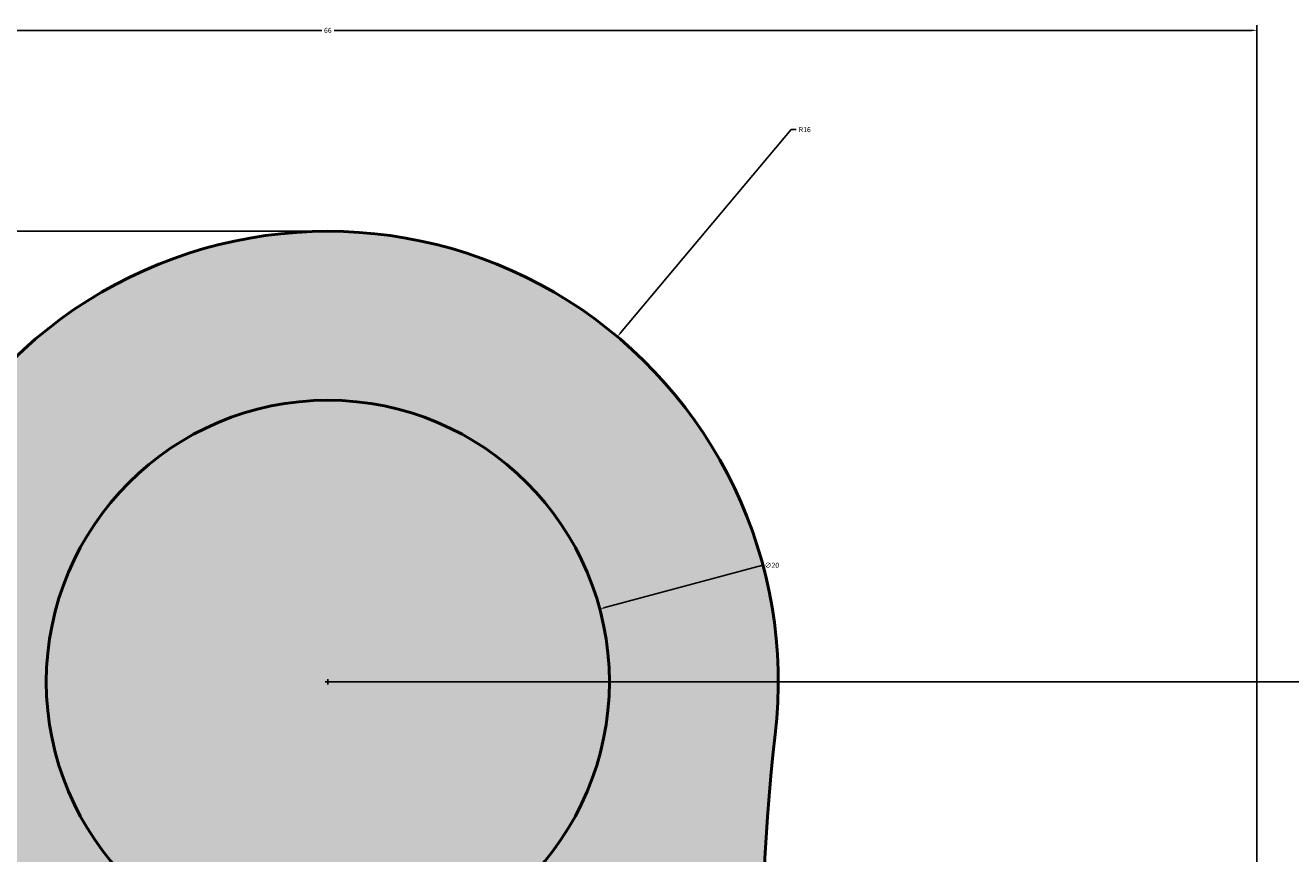
# Model space of a CAD drawing. Units: inches. Extents: x -13 to 107, y -48 to 102.
# Tile 12 of 13: x 17 to 62, y 72 to 102. Entities that reach past the tile are written whole.
import ezdxf

# ---------------------------------------------------------------- set-up
doc = ezdxf.new("R2010")
doc.units = ezdxf.units.IN
doc.header["$MEASUREMENT"] = 0
for name, color, linetype, lineweight in [('M-DIMS', 2, 'Continuous', 18), ('M-HATC', 8, 'Continuous', 18), ('M-OUTL', 7, 'Continuous', 50)]:
    doc.layers.add(name, color=color, linetype=linetype, lineweight=lineweight)
doc.styles.get("Standard").update_dxf_attribs({"font": 'arial.ttf'})
doc.dimstyles.get("Standard").update_dxf_attribs({"dimtxt": 0.18, "dimasz": 0.18, "dimexe": 0.18, "dimexo": 0.0625, "dimgap": 0.09, "dimtad": 0, "dimtih": 1, "dimtoh": 1, "dimdec": 4, "dimzin": 0, "dimdsep": 46, "dimtxsty": 'Standard', "dimcen": 0.09, "dimadec": 0, "dimazin": 0, "dimtfac": 1, "dimtdec": 4, "dimtofl": 0, "dimtmove": 0, "dimatfit": 3, "dimfxl": 1, "dimtolj": 1, "dimtzin": 0, "dimarcsym": 0})

# ---------------------------------------------------------------- blocks, each defined once
blk = doc.blocks.new('*D1')
at = {"layer": 'Defpoints', "color": 0, "transparency": 16777216}
for p in [(60.544, 101.543), (-5.45, 13.883), (60.544, 13.883)]:
    blk.add_point(p, dxfattribs=at)
at = {"layer": 'M-DIMS', "color": 0, "lineweight": -2, "transparency": 16777216}
for p, q in [((-5.45, 13.945), (-5.45, 101.723)), ((60.544, 13.945), (60.544, 101.723)), ((-5.27, 101.543), (27.328, 101.543)), ((60.364, 101.543), (27.766, 101.543))]:
    blk.add_line(p, q, dxfattribs=at)
at = {"layer": 'M-DIMS', "color": 0, "transparency": 16777216}
for points in [[(-5.27, 101.573), (-5.27, 101.513), (-5.45, 101.543)], [(60.364, 101.573), (60.364, 101.513), (60.544, 101.543)]]:
    blk.add_solid(points, dxfattribs=at)
at = {"layer": 'M-DIMS', "color": 0, "transparency": 16777216, "insert": (27.547, 101.543), "char_height": 0.18, "attachment_point": 5}
blk.add_mtext('\\A1;66', dxfattribs=at)
blk = doc.blocks.new('*D2')
at = {"layer": 'Defpoints', "color": 0, "transparency": 16777216}
for p in [(-12.585, 94.408), (27.547, 94.408), (27.547, -46.592)]:
    blk.add_point(p, dxfattribs=at)
at = {"layer": 'M-DIMS', "color": 0, "lineweight": -2, "transparency": 16777216}
for p, q in [((27.484, 94.408), (-12.765, 94.408)), ((-12.585, 94.228), (-12.585, 24.088)), ((-12.585, -46.412), (-12.585, 23.727)), ((27.484, -46.592), (-12.765, -46.592))]:
    blk.add_line(p, q, dxfattribs=at)
at = {"layer": 'M-DIMS', "color": 0, "transparency": 16777216}
for points in [[(-12.615, 94.228), (-12.555, 94.228), (-12.585, 94.408)], [(-12.615, -46.412), (-12.555, -46.412), (-12.585, -46.592)]]:
    blk.add_solid(points, dxfattribs=at)
at = {"layer": 'M-DIMS', "color": 0, "transparency": 16777216, "insert": (-12.585, 23.908), "char_height": 0.18, "attachment_point": 5}
blk.add_mtext('\\A1;141', dxfattribs=at)
blk = doc.blocks.new('*D4')
at = {"layer": 'Defpoints', "color": 0, "transparency": 16777216}
for p in [(27.547, 78.408), (67.679, 78.408), (27.547, 13.408)]:
    blk.add_point(p, dxfattribs=at)
at = {"layer": 'M-DIMS', "color": 0, "lineweight": -2, "transparency": 16777216}
for p, q in [((27.609, 78.408), (67.859, 78.408)), ((67.679, 78.228), (67.679, 46.09)), ((67.679, 13.588), (67.679, 45.726)), ((27.609, 13.408), (67.859, 13.408))]:
    blk.add_line(p, q, dxfattribs=at)
at = {"layer": 'M-DIMS', "color": 0, "transparency": 16777216}
for points in [[(67.649, 78.228), (67.709, 78.228), (67.679, 78.408)], [(67.649, 13.588), (67.709, 13.588), (67.679, 13.408)]]:
    blk.add_solid(points, dxfattribs=at)
at = {"layer": 'M-DIMS', "color": 0, "transparency": 16777216, "insert": (67.679, 45.908), "char_height": 0.18, "attachment_point": 5}
blk.add_mtext('\\A1;65', dxfattribs=at)
blk = doc.blocks.new('*D6')
at = {"layer": 'Defpoints', "color": 0, "transparency": 16777216}
for p in [(37.832, 90.665), (27.547, 78.408)]:
    blk.add_point(p, dxfattribs=at)
at = {"layer": 'M-DIMS', "color": 0, "lineweight": -2, "transparency": 16777216}
for p, q in [((44.002, 98.019), (37.947, 90.802)), ((44.182, 98.019), (44.002, 98.019)), ((27.457, 78.408), (27.637, 78.408)), ((27.547, 78.318), (27.547, 78.498))]:
    blk.add_line(p, q, dxfattribs=at)
at = {"layer": 'M-DIMS', "color": 0, "transparency": 16777216}
blk.add_solid([(37.924, 90.822), (37.97, 90.783), (37.832, 90.665)], dxfattribs=at)
at = {"layer": 'M-DIMS', "color": 0, "transparency": 16777216, "insert": (44.487, 98.019), "char_height": 0.18, "attachment_point": 5}
blk.add_mtext('\\A1;R16', dxfattribs=at)
blk = doc.blocks.new('*D7')
at = {"layer": 'Defpoints', "color": 0, "transparency": 16777216}
for p in [(37.206, 80.996), (17.888, 75.82)]:
    blk.add_point(p, dxfattribs=at)
at = {"layer": 'M-DIMS', "color": 0, "lineweight": -2, "transparency": 16777216}
for p, q in [((43.002, 82.549), (37.38, 81.042)), ((27.457, 78.408), (27.637, 78.408)), ((27.547, 78.318), (27.547, 78.498))]:
    blk.add_line(p, q, dxfattribs=at)
at = {"layer": 'M-DIMS', "color": 0, "transparency": 16777216}
blk.add_solid([(37.372, 81.071), (37.388, 81.013), (37.206, 80.996)], dxfattribs=at)
at = {"layer": 'M-DIMS', "color": 0, "transparency": 16777216, "insert": (43.318, 82.549), "char_height": 0.18, "attachment_point": 5}
blk.add_mtext('\\A1;∅20', dxfattribs=at)

msp = doc.modelspace()

# ---------------------------------------------------------------- hatches: boundary and pattern name
at = {"layer": 'M-HATC'}
h = msp.add_hatch(color=256, dxfattribs=at)
h.set_gradient(color1=(88, 186, 72), color2=(241, 235, 31), tint=1)
h.paths.add_polyline_path([(45.86, -14.044, 0.420873), (54.577, 32.339, -0.184081), (43.437, 76.537, 1.124637), (11.657, 76.537, -0.184081), (0.517, 32.339, 0.420873), (9.234, -14.044, -0.304084), (17.743, -34.622, 1.220926), (37.351, -34.622, -0.304084)])
h.paths.add_polyline_path([(33.479, -5.692, 0.859727), (21.615, -5.692, -0.111692), (13.972, -1.28, 0.859727), (8.04, 8.995, -0.111692), (8.04, 17.82, 0.859727), (13.972, 28.095, -0.111692), (21.615, 32.508, 0.859727), (33.479, 32.508, -0.111692), (41.122, 28.095, 0.859727), (47.054, 17.82, -0.111692), (47.054, 8.995, 0.859727), (41.122, -1.28, -0.111692)], flags=16)
h.paths.add_polyline_path([(32.547, -36.592, -1), (22.547, -36.592, -1)], flags=16)
h.paths.add_polyline_path([(17.547, 78.408, -1), (37.547, 78.408, -1)], flags=16)
h = msp.add_hatch(color=256, dxfattribs=at)
h.set_gradient(color1=(0, 0, 255), tint=1)
h.paths.add_polyline_path([(47.054, 8.995, 0.111692), (47.054, 17.82, -0.859727), (41.122, 28.095, 0.111692), (33.479, 32.508, -0.859727), (21.615, 32.508, 0.111692), (13.972, 28.095, -0.859727), (8.04, 17.82, 0.111692), (8.04, 8.995, -0.859727), (13.972, -1.28, 0.111692), (21.615, -5.692, -0.859727), (33.479, -5.692, 0.111692), (41.122, -1.28, -0.859727)])
h.paths.add_polyline_path([(37.547, 78.408, 1), (17.547, 78.408, 1)])
h.paths.add_polyline_path([(32.547, -36.592, 1), (22.547, -36.592, 1)])

# ---------------------------------------------------------------- linework, layer by layer
at = {"layer": 'M-OUTL'}
msp.add_circle((27.547, 78.408), 10, dxfattribs=at)
for centre, radius, start, end in [((27.547, 78.408), 16, 353.2854, 186.7146), ((106.998, 69.054), 64, 173.28544, 215.00666)]:
    msp.add_arc(centre, radius, start, end, dxfattribs=at)

# ---------------------------------------------------------------- dimensions: what is measured, and where the dimension line sits
at = {"layer": 'M-DIMS'}
dim = msp.add_linear_dim(base=(60.544, 101.543), p1=(-5.45, 13.883), p2=(60.544, 13.883), dimstyle='Standard', override={"dimdec": 0, "dimlfac": 1, "dimrnd": 0, "dimzin": 0, "dimdsep": 46, "dimlunit": 2}, dxfattribs=at)
dim.commit()
dim.dimension.update_dxf_attribs({"geometry": '*D1', "text_midpoint": (27.547, 101.543)})
dim = msp.add_radius_dim(center=(27.547, 78.408), mpoint=(37.832, 90.665), dimstyle='Standard', override={"dimdec": 0, "dimlfac": 1, "dimrnd": 0, "dimzin": 0, "dimdsep": 46, "dimlunit": 2}, dxfattribs=at)
dim.commit()
dim.dimension.update_dxf_attribs({"geometry": '*D6', "text_midpoint": (44.487, 98.019), "dimtype": 164})
for base, p1, p2, picture, middle in [((-12.585, 94.408), (27.547, -46.592), (27.547, 94.408), '*D2', (-12.585, 23.908)), ((67.679, 78.408), (27.547, 13.408), (27.547, 78.408), '*D4', (67.679, 45.908))]:
    dim = msp.add_linear_dim(base=base, p1=p1, p2=p2, angle=90, dimstyle='Standard', override={"dimdec": 0, "dimlfac": 1, "dimrnd": 0, "dimzin": 0, "dimdsep": 46, "dimlunit": 2}, dxfattribs=at)
    dim.commit()
    dim.dimension.update_dxf_attribs({"geometry": picture, "text_midpoint": middle})
dim = msp.add_diameter_dim_2p(p1=(17.888, 75.82), p2=(37.206, 80.996), dimstyle='Standard', override={"dimdec": 0, "dimlfac": 1, "dimrnd": 0, "dimzin": 0, "dimdsep": 46, "dimlunit": 2}, dxfattribs=at)
dim.commit()
dim.dimension.update_dxf_attribs({"geometry": '*D7', "text_midpoint": (43.002, 82.549), "dimtype": 163})

doc.saveas('drawing.dxf')
